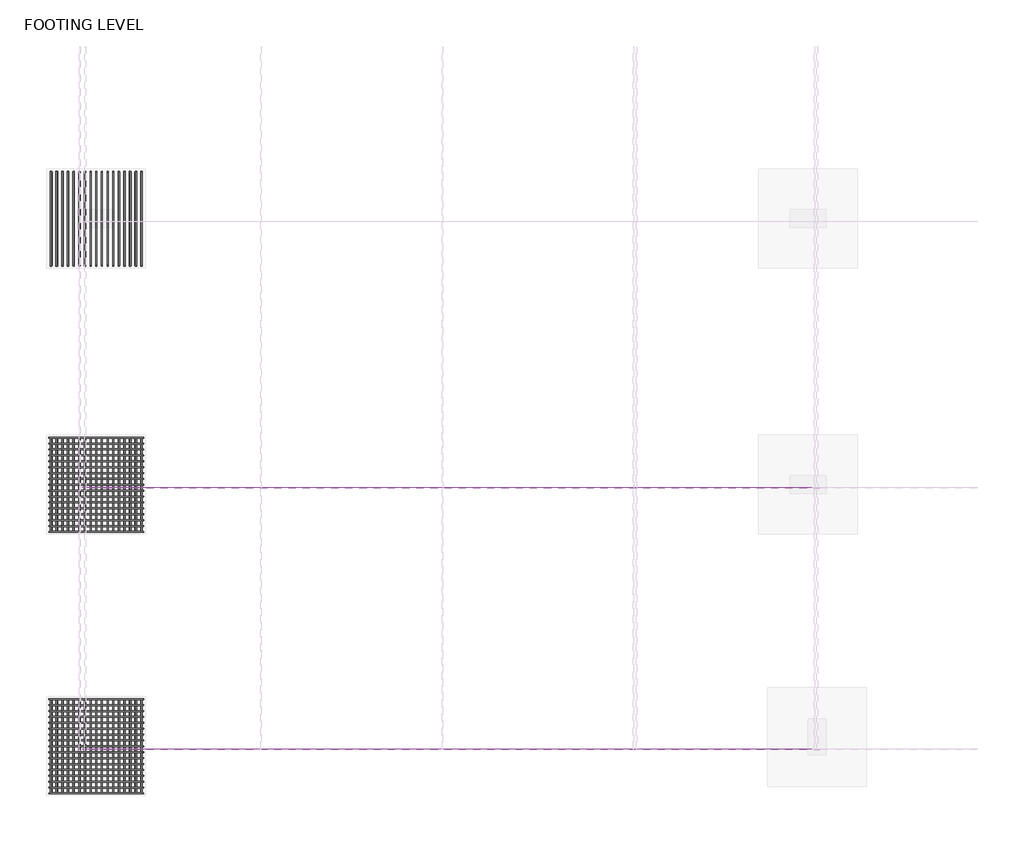
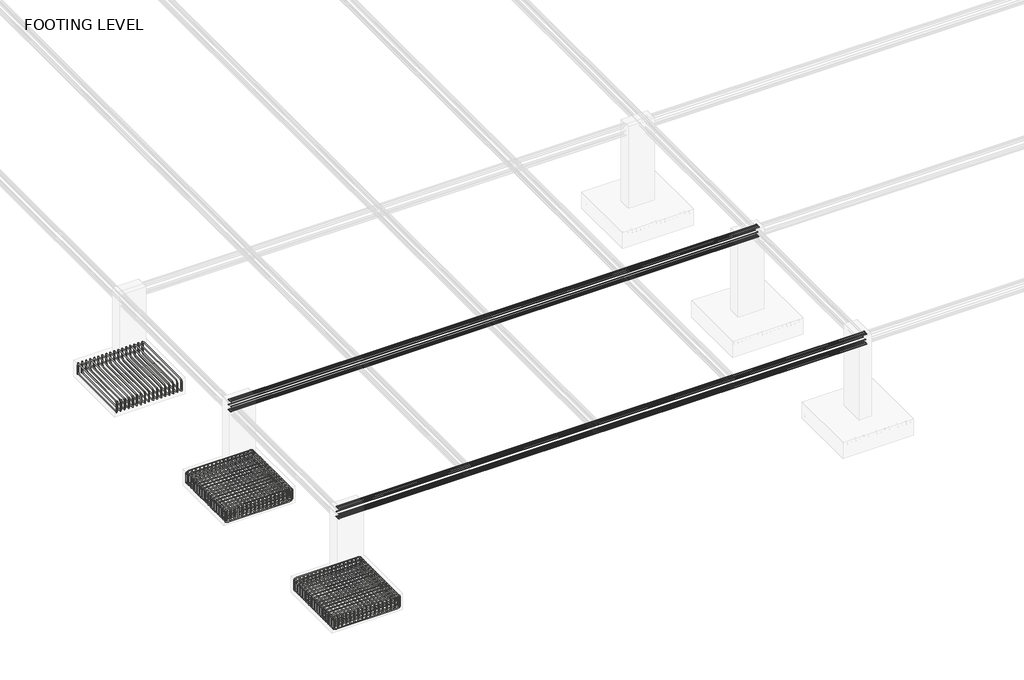
# One storey, part 3 of 19: 16 reinforcing bars.
"""IFC4 building model written with IfcOpenShell, lengths in millimetres."""

from ifc_helpers import new_model, si_unit, point, frame, origin, place, context, project, spatial, polyline, circle_curve, trimmed, segment, composite_curve, source, transform, mapped, element, save
from ifc_brep_helpers import swept_disk

model = new_model("IFC4")

# Units and contexts
model_context = context("Model", 3, world=origin())
ifc_project = project(units=[si_unit("LENGTHUNIT", "METRE", prefix="MILLI")], contexts=[model_context])

# Site, building, storey
site = spatial("IfcSite", under=ifc_project)
building = spatial("IfcBuilding", under=site)
storey = spatial("IfcBuildingStorey", under=building, Name="FOOTING LEVEL", Elevation=-3048.0)

# Reinforcing bars
placement = place(None, origin())
reinforcing_bar_shape = source(origin(), model_context, "Body", "SolidModel", [
    swept_disk(composite_curve([segment(polyline([(-17920.0723448, -29246.9205555, -3148.0), (-17920.0723448, -29246.9205555, -3470.1)]), True, "CONTINUOUS"), segment(trimmed(circle_curve(frame((-17920.0723448, -29156.7205555, -3470.1), z_axis=(1.0, 0.0, 0.0), x_axis=(0.0, -90.20000000000073, 0.0)), 90.2), [point((-17920.0723448, -29246.9205555, -3470.1))], [point((-17920.0723448, -29156.7205555, -3560.3))], True, "CARTESIAN"), True, "CONTINUOUS"), segment(polyline([(-17920.0723448, -29156.7205555, -3560.3), (-17920.0723448, -26962.5205555, -3560.3)]), True, "CONTINUOUS"), segment(trimmed(circle_curve(frame((-17920.0723448, -26962.5205555, -3470.1), z_axis=(1.0, 0.0, 0.0), x_axis=(0.0, 0.0, -90.20000000000027)), 90.2), [point((-17920.0723448, -26962.5205555, -3560.3))], [point((-17920.0723448, -26872.3205555, -3470.1))], True, "CARTESIAN"), True, "CONTINUOUS"), segment(polyline([(-17920.0723448, -26872.3205555, -3470.1), (-17920.0723448, -26872.3205555, -3148.0)]), True, "CONTINUOUS")], self_intersect=False), 12.7),
])
element("IfcReinforcingBar", 1, at=placement, inside=storey, context=model_context, shape_type="MappedRepresentation", body=[
    mapped(reinforcing_bar_shape, transform((0.0, 0.0, 0.0), x_axis=(1.0, 0.0, 0.0), y_axis=(0.0, 1.0, 0.0), z_axis=(0.0, 0.0, 1.0))),
    mapped(reinforcing_bar_shape, transform((140.8090411, 0.0, 0.0), x_axis=(1.0, 0.0, 0.0), y_axis=(0.0, 1.0, 0.0), z_axis=(0.0, 0.0, 1.0))),
    mapped(reinforcing_bar_shape, transform((281.6180821, 0.0, 0.0), x_axis=(1.0, 0.0, 0.0), y_axis=(0.0, 1.0, 0.0), z_axis=(0.0, 0.0, 1.0))),
    mapped(reinforcing_bar_shape, transform((422.4271232, 0.0, 0.0), x_axis=(1.0, 0.0, 0.0), y_axis=(0.0, 1.0, 0.0), z_axis=(0.0, 0.0, 1.0))),
    mapped(reinforcing_bar_shape, transform((563.2361643, 0.0, 0.0), x_axis=(1.0, 0.0, 0.0), y_axis=(0.0, 1.0, 0.0), z_axis=(0.0, 0.0, 1.0))),
    mapped(reinforcing_bar_shape, transform((704.0452054, 0.0, 0.0), x_axis=(1.0, 0.0, 0.0), y_axis=(0.0, 1.0, 0.0), z_axis=(0.0, 0.0, 1.0))),
    mapped(reinforcing_bar_shape, transform((844.8542464, 0.0, 0.0), x_axis=(1.0, 0.0, 0.0), y_axis=(0.0, 1.0, 0.0), z_axis=(0.0, 0.0, 1.0))),
    mapped(reinforcing_bar_shape, transform((985.6632875, 0.0, 0.0), x_axis=(1.0, 0.0, 0.0), y_axis=(0.0, 1.0, 0.0), z_axis=(0.0, 0.0, 1.0))),
    mapped(reinforcing_bar_shape, transform((1126.4723286, 0.0, 0.0), x_axis=(1.0, 0.0, 0.0), y_axis=(0.0, 1.0, 0.0), z_axis=(0.0, 0.0, 1.0))),
    mapped(reinforcing_bar_shape, transform((1267.2813697, 0.0, 0.0), x_axis=(1.0, 0.0, 0.0), y_axis=(0.0, 1.0, 0.0), z_axis=(0.0, 0.0, 1.0))),
    mapped(reinforcing_bar_shape, transform((1408.0904107, 0.0, 0.0), x_axis=(1.0, 0.0, 0.0), y_axis=(0.0, 1.0, 0.0), z_axis=(0.0, 0.0, 1.0))),
    mapped(reinforcing_bar_shape, transform((1548.8994518, 0.0, 0.0), x_axis=(1.0, 0.0, 0.0), y_axis=(0.0, 1.0, 0.0), z_axis=(0.0, 0.0, 1.0))),
    mapped(reinforcing_bar_shape, transform((1689.7084929, 0.0, 0.0), x_axis=(1.0, 0.0, 0.0), y_axis=(0.0, 1.0, 0.0), z_axis=(0.0, 0.0, 1.0))),
    mapped(reinforcing_bar_shape, transform((1830.517534, 0.0, 0.0), x_axis=(1.0, 0.0, 0.0), y_axis=(0.0, 1.0, 0.0), z_axis=(0.0, 0.0, 1.0))),
    mapped(reinforcing_bar_shape, transform((1971.326575, 0.0, 0.0), x_axis=(1.0, 0.0, 0.0), y_axis=(0.0, 1.0, 0.0), z_axis=(0.0, 0.0, 1.0))),
    mapped(reinforcing_bar_shape, transform((2112.1356161, 0.0, 0.0), x_axis=(1.0, 0.0, 0.0), y_axis=(0.0, 1.0, 0.0), z_axis=(0.0, 0.0, 1.0))),
    mapped(reinforcing_bar_shape, transform((2252.9446572, 0.0, 0.0), x_axis=(1.0, 0.0, 0.0), y_axis=(0.0, 1.0, 0.0), z_axis=(0.0, 0.0, 1.0))),
])
reinforcing_bar_2_shape = source(origin(), model_context, "Body", "SolidModel", [
    swept_disk(composite_curve([segment(polyline([(-15644.6802955, -29246.9205555, -3548.0), (-15644.6802955, -29246.9205555, -3225.9)]), True, "CONTINUOUS"), segment(trimmed(circle_curve(frame((-15644.6802955, -29156.7205555, -3225.9), z_axis=(-1.0, 0.0, 0.0), x_axis=(0.0, -90.20000000000073, 0.0)), 90.2), [point((-15644.6802955, -29246.9205555, -3225.9))], [point((-15644.6802955, -29156.7205555, -3135.7))], True, "CARTESIAN"), True, "CONTINUOUS"), segment(polyline([(-15644.6802955, -29156.7205555, -3135.7), (-15644.6802955, -26962.5205555, -3135.7)]), True, "CONTINUOUS"), segment(trimmed(circle_curve(frame((-15644.6802955, -26962.5205555, -3225.9), z_axis=(-1.0, 0.0, 0.0), x_axis=(0.0, 0.0, 90.20000000000027)), 90.2), [point((-15644.6802955, -26962.5205555, -3135.7))], [point((-15644.6802955, -26872.3205555, -3225.9))], True, "CARTESIAN"), True, "CONTINUOUS"), segment(polyline([(-15644.6802955, -26872.3205555, -3225.9), (-15644.6802955, -26872.3205555, -3548.0)]), True, "CONTINUOUS")], self_intersect=False), 12.7),
])
element("IfcReinforcingBar", 2, at=placement, inside=storey, context=model_context, shape_type="MappedRepresentation", body=[
    mapped(reinforcing_bar_2_shape, transform((0.0, 0.0, 0.0), x_axis=(1.0, 0.0, 0.0), y_axis=(0.0, 1.0, 0.0), z_axis=(0.0, 0.0, 1.0))),
    mapped(reinforcing_bar_2_shape, transform((-143.8496077, 0.0, 0.0), x_axis=(1.0, 0.0, 0.0), y_axis=(0.0, 1.0, 0.0), z_axis=(0.0, 0.0, 1.0))),
    mapped(reinforcing_bar_2_shape, transform((-287.6992155, 0.0, 0.0), x_axis=(1.0, 0.0, 0.0), y_axis=(0.0, 1.0, 0.0), z_axis=(0.0, 0.0, 1.0))),
    mapped(reinforcing_bar_2_shape, transform((-431.5488232, 0.0, 0.0), x_axis=(1.0, 0.0, 0.0), y_axis=(0.0, 1.0, 0.0), z_axis=(0.0, 0.0, 1.0))),
    mapped(reinforcing_bar_2_shape, transform((-575.398431, 0.0, 0.0), x_axis=(1.0, 0.0, 0.0), y_axis=(0.0, 1.0, 0.0), z_axis=(0.0, 0.0, 1.0))),
    mapped(reinforcing_bar_2_shape, transform((-719.2480387, 0.0, 0.0), x_axis=(1.0, 0.0, 0.0), y_axis=(0.0, 1.0, 0.0), z_axis=(0.0, 0.0, 1.0))),
    mapped(reinforcing_bar_2_shape, transform((-863.0976465, 0.0, 0.0), x_axis=(1.0, 0.0, 0.0), y_axis=(0.0, 1.0, 0.0), z_axis=(0.0, 0.0, 1.0))),
    mapped(reinforcing_bar_2_shape, transform((-1006.9472542, 0.0, 0.0), x_axis=(1.0, 0.0, 0.0), y_axis=(0.0, 1.0, 0.0), z_axis=(0.0, 0.0, 1.0))),
    mapped(reinforcing_bar_2_shape, transform((-1150.796862, 0.0, 0.0), x_axis=(1.0, 0.0, 0.0), y_axis=(0.0, 1.0, 0.0), z_axis=(0.0, 0.0, 1.0))),
    mapped(reinforcing_bar_2_shape, transform((-1294.6464697, 0.0, 0.0), x_axis=(1.0, 0.0, 0.0), y_axis=(0.0, 1.0, 0.0), z_axis=(0.0, 0.0, 1.0))),
    mapped(reinforcing_bar_2_shape, transform((-1438.4960775, 0.0, 0.0), x_axis=(1.0, 0.0, 0.0), y_axis=(0.0, 1.0, 0.0), z_axis=(0.0, 0.0, 1.0))),
    mapped(reinforcing_bar_2_shape, transform((-1582.3456852, 0.0, 0.0), x_axis=(1.0, 0.0, 0.0), y_axis=(0.0, 1.0, 0.0), z_axis=(0.0, 0.0, 1.0))),
    mapped(reinforcing_bar_2_shape, transform((-1726.195293, 0.0, 0.0), x_axis=(1.0, 0.0, 0.0), y_axis=(0.0, 1.0, 0.0), z_axis=(0.0, 0.0, 1.0))),
    mapped(reinforcing_bar_2_shape, transform((-1870.0449007, 0.0, 0.0), x_axis=(1.0, 0.0, 0.0), y_axis=(0.0, 1.0, 0.0), z_axis=(0.0, 0.0, 1.0))),
    mapped(reinforcing_bar_2_shape, transform((-2013.8945085, 0.0, 0.0), x_axis=(1.0, 0.0, 0.0), y_axis=(0.0, 1.0, 0.0), z_axis=(0.0, 0.0, 1.0))),
    mapped(reinforcing_bar_2_shape, transform((-2157.7441162, 0.0, 0.0), x_axis=(1.0, 0.0, 0.0), y_axis=(0.0, 1.0, 0.0), z_axis=(0.0, 0.0, 1.0))),
    mapped(reinforcing_bar_2_shape, transform((-2301.5937239, 0.0, 0.0), x_axis=(1.0, 0.0, 0.0), y_axis=(0.0, 1.0, 0.0), z_axis=(0.0, 0.0, 1.0))),
])
reinforcing_bar_3_shape = source(origin(), model_context, "Body", "SolidModel", [
    swept_disk(composite_curve([segment(polyline([(-17985.6412437, -26872.3205555, -3173.0), (-17985.6412437, -26872.3205555, -3495.1)]), True, "CONTINUOUS"), segment(trimmed(circle_curve(frame((-17895.4412437, -26872.3205555, -3495.1), z_axis=(0.0, -1.0, 0.0), x_axis=(-90.20000000000073, 0.0, 0.0)), 90.2), [point((-17985.6412437, -26872.3205555, -3495.1))], [point((-17895.4412437, -26872.3205555, -3585.3))], True, "CARTESIAN"), True, "CONTINUOUS"), segment(polyline([(-17895.4412437, -26872.3205555, -3585.3), (-15701.2412437, -26872.3205555, -3585.3)]), True, "CONTINUOUS"), segment(trimmed(circle_curve(frame((-15701.2412437, -26872.3205555, -3495.1), z_axis=(0.0, -1.0, 0.0), x_axis=(0.0, 0.0, -90.20000000000027)), 90.2), [point((-15701.2412437, -26872.3205555, -3585.3))], [point((-15611.0412437, -26872.3205555, -3495.1))], True, "CARTESIAN"), True, "CONTINUOUS"), segment(polyline([(-15611.0412437, -26872.3205555, -3495.1), (-15611.0412437, -26872.3205555, -3173.0)]), True, "CONTINUOUS")], self_intersect=False), 12.7),
])
element("IfcReinforcingBar", 3, at=placement, inside=storey, context=model_context, shape_type="MappedRepresentation", body=[
    mapped(reinforcing_bar_3_shape, transform((0.0, 0.0, 0.0), x_axis=(1.0, 0.0, 0.0), y_axis=(0.0, 1.0, 0.0), z_axis=(0.0, 0.0, 1.0))),
    mapped(reinforcing_bar_3_shape, transform((0.0, -148.4125, 0.0), x_axis=(1.0, 0.0, 0.0), y_axis=(0.0, 1.0, 0.0), z_axis=(0.0, 0.0, 1.0))),
    mapped(reinforcing_bar_3_shape, transform((0.0, -296.825, 0.0), x_axis=(1.0, 0.0, 0.0), y_axis=(0.0, 1.0, 0.0), z_axis=(0.0, 0.0, 1.0))),
    mapped(reinforcing_bar_3_shape, transform((0.0, -445.2375, 0.0), x_axis=(1.0, 0.0, 0.0), y_axis=(0.0, 1.0, 0.0), z_axis=(0.0, 0.0, 1.0))),
    mapped(reinforcing_bar_3_shape, transform((0.0, -593.65, 0.0), x_axis=(1.0, 0.0, 0.0), y_axis=(0.0, 1.0, 0.0), z_axis=(0.0, 0.0, 1.0))),
    mapped(reinforcing_bar_3_shape, transform((0.0, -742.0625, 0.0), x_axis=(1.0, 0.0, 0.0), y_axis=(0.0, 1.0, 0.0), z_axis=(0.0, 0.0, 1.0))),
    mapped(reinforcing_bar_3_shape, transform((0.0, -890.475, 0.0), x_axis=(1.0, 0.0, 0.0), y_axis=(0.0, 1.0, 0.0), z_axis=(0.0, 0.0, 1.0))),
    mapped(reinforcing_bar_3_shape, transform((0.0, -1038.8875, 0.0), x_axis=(1.0, 0.0, 0.0), y_axis=(0.0, 1.0, 0.0), z_axis=(0.0, 0.0, 1.0))),
    mapped(reinforcing_bar_3_shape, transform((0.0, -1187.3, 0.0), x_axis=(1.0, 0.0, 0.0), y_axis=(0.0, 1.0, 0.0), z_axis=(0.0, 0.0, 1.0))),
    mapped(reinforcing_bar_3_shape, transform((0.0, -1335.7125, 0.0), x_axis=(1.0, 0.0, 0.0), y_axis=(0.0, 1.0, 0.0), z_axis=(0.0, 0.0, 1.0))),
    mapped(reinforcing_bar_3_shape, transform((0.0, -1484.125, 0.0), x_axis=(1.0, 0.0, 0.0), y_axis=(0.0, 1.0, 0.0), z_axis=(0.0, 0.0, 1.0))),
    mapped(reinforcing_bar_3_shape, transform((0.0, -1632.5375, 0.0), x_axis=(1.0, 0.0, 0.0), y_axis=(0.0, 1.0, 0.0), z_axis=(0.0, 0.0, 1.0))),
    mapped(reinforcing_bar_3_shape, transform((0.0, -1780.95, 0.0), x_axis=(1.0, 0.0, 0.0), y_axis=(0.0, 1.0, 0.0), z_axis=(0.0, 0.0, 1.0))),
    mapped(reinforcing_bar_3_shape, transform((0.0, -1929.3625, 0.0), x_axis=(1.0, 0.0, 0.0), y_axis=(0.0, 1.0, 0.0), z_axis=(0.0, 0.0, 1.0))),
    mapped(reinforcing_bar_3_shape, transform((0.0, -2077.775, 0.0), x_axis=(1.0, 0.0, 0.0), y_axis=(0.0, 1.0, 0.0), z_axis=(0.0, 0.0, 1.0))),
    mapped(reinforcing_bar_3_shape, transform((0.0, -2226.1875, 0.0), x_axis=(1.0, 0.0, 0.0), y_axis=(0.0, 1.0, 0.0), z_axis=(0.0, 0.0, 1.0))),
    mapped(reinforcing_bar_3_shape, transform((0.0, -2374.6, 0.0), x_axis=(1.0, 0.0, 0.0), y_axis=(0.0, 1.0, 0.0), z_axis=(0.0, 0.0, 1.0))),
])
reinforcing_bar_4_shape = source(origin(), model_context, "Body", "SolidModel", [
    swept_disk(composite_curve([segment(polyline([(-15611.0412437, -26872.3205555, -3523.0), (-15611.0412437, -26872.3205555, -3200.9)]), True, "CONTINUOUS"), segment(trimmed(circle_curve(frame((-15701.2412437, -26872.3205555, -3200.9), z_axis=(0.0, -1.0, 0.0), x_axis=(90.20000000000073, 0.0, 0.0)), 90.2), [point((-15611.0412437, -26872.3205555, -3200.9))], [point((-15701.2412437, -26872.3205555, -3110.7))], True, "CARTESIAN"), True, "CONTINUOUS"), segment(polyline([(-15701.2412437, -26872.3205555, -3110.7), (-17895.4412437, -26872.3205555, -3110.7)]), True, "CONTINUOUS"), segment(trimmed(circle_curve(frame((-17895.4412437, -26872.3205555, -3200.9), z_axis=(0.0, -1.0, 0.0), x_axis=(0.0, 0.0, 90.20000000000027)), 90.2), [point((-17895.4412437, -26872.3205555, -3110.7))], [point((-17985.6412437, -26872.3205555, -3200.9))], True, "CARTESIAN"), True, "CONTINUOUS"), segment(polyline([(-17985.6412437, -26872.3205555, -3200.9), (-17985.6412437, -26872.3205555, -3523.0)]), True, "CONTINUOUS")], self_intersect=False), 12.7),
])
element("IfcReinforcingBar", 4, at=placement, inside=storey, context=model_context, shape_type="MappedRepresentation", body=[
    mapped(reinforcing_bar_4_shape, transform((0.0, 0.0, 0.0), x_axis=(1.0, 0.0, 0.0), y_axis=(0.0, 1.0, 0.0), z_axis=(0.0, 0.0, 1.0))),
    mapped(reinforcing_bar_4_shape, transform((0.0, -148.4125, 0.0), x_axis=(1.0, 0.0, 0.0), y_axis=(0.0, 1.0, 0.0), z_axis=(0.0, 0.0, 1.0))),
    mapped(reinforcing_bar_4_shape, transform((0.0, -296.825, 0.0), x_axis=(1.0, 0.0, 0.0), y_axis=(0.0, 1.0, 0.0), z_axis=(0.0, 0.0, 1.0))),
    mapped(reinforcing_bar_4_shape, transform((0.0, -445.2375, 0.0), x_axis=(1.0, 0.0, 0.0), y_axis=(0.0, 1.0, 0.0), z_axis=(0.0, 0.0, 1.0))),
    mapped(reinforcing_bar_4_shape, transform((0.0, -593.65, 0.0), x_axis=(1.0, 0.0, 0.0), y_axis=(0.0, 1.0, 0.0), z_axis=(0.0, 0.0, 1.0))),
    mapped(reinforcing_bar_4_shape, transform((0.0, -742.0625, 0.0), x_axis=(1.0, 0.0, 0.0), y_axis=(0.0, 1.0, 0.0), z_axis=(0.0, 0.0, 1.0))),
    mapped(reinforcing_bar_4_shape, transform((0.0, -890.475, 0.0), x_axis=(1.0, 0.0, 0.0), y_axis=(0.0, 1.0, 0.0), z_axis=(0.0, 0.0, 1.0))),
    mapped(reinforcing_bar_4_shape, transform((0.0, -1038.8875, 0.0), x_axis=(1.0, 0.0, 0.0), y_axis=(0.0, 1.0, 0.0), z_axis=(0.0, 0.0, 1.0))),
    mapped(reinforcing_bar_4_shape, transform((0.0, -1187.3, 0.0), x_axis=(1.0, 0.0, 0.0), y_axis=(0.0, 1.0, 0.0), z_axis=(0.0, 0.0, 1.0))),
    mapped(reinforcing_bar_4_shape, transform((0.0, -1335.7125, 0.0), x_axis=(1.0, 0.0, 0.0), y_axis=(0.0, 1.0, 0.0), z_axis=(0.0, 0.0, 1.0))),
    mapped(reinforcing_bar_4_shape, transform((0.0, -1484.125, 0.0), x_axis=(1.0, 0.0, 0.0), y_axis=(0.0, 1.0, 0.0), z_axis=(0.0, 0.0, 1.0))),
    mapped(reinforcing_bar_4_shape, transform((0.0, -1632.5375, 0.0), x_axis=(1.0, 0.0, 0.0), y_axis=(0.0, 1.0, 0.0), z_axis=(0.0, 0.0, 1.0))),
    mapped(reinforcing_bar_4_shape, transform((0.0, -1780.95, 0.0), x_axis=(1.0, 0.0, 0.0), y_axis=(0.0, 1.0, 0.0), z_axis=(0.0, 0.0, 1.0))),
    mapped(reinforcing_bar_4_shape, transform((0.0, -1929.3625, 0.0), x_axis=(1.0, 0.0, 0.0), y_axis=(0.0, 1.0, 0.0), z_axis=(0.0, 0.0, 1.0))),
    mapped(reinforcing_bar_4_shape, transform((0.0, -2077.775, 0.0), x_axis=(1.0, 0.0, 0.0), y_axis=(0.0, 1.0, 0.0), z_axis=(0.0, 0.0, 1.0))),
    mapped(reinforcing_bar_4_shape, transform((0.0, -2226.1875, 0.0), x_axis=(1.0, 0.0, 0.0), y_axis=(0.0, 1.0, 0.0), z_axis=(0.0, 0.0, 1.0))),
    mapped(reinforcing_bar_4_shape, transform((0.0, -2374.6, 0.0), x_axis=(1.0, 0.0, 0.0), y_axis=(0.0, 1.0, 0.0), z_axis=(0.0, 0.0, 1.0))),
])
reinforcing_bar_5_shape = source(origin(), model_context, "Body", "SolidModel", [
    swept_disk(composite_curve([segment(polyline([(-17920.0723448, -22655.6205555, -3148.0), (-17920.0723448, -22655.6205555, -3470.1)]), True, "CONTINUOUS"), segment(trimmed(circle_curve(frame((-17920.0723448, -22565.4205555, -3470.1), z_axis=(1.0, 0.0, 0.0), x_axis=(0.0, -90.20000000000073, 0.0)), 90.2), [point((-17920.0723448, -22655.6205555, -3470.1))], [point((-17920.0723448, -22565.4205555, -3560.3))], True, "CARTESIAN"), True, "CONTINUOUS"), segment(polyline([(-17920.0723448, -22565.4205555, -3560.3), (-17920.0723448, -20371.2205555, -3560.3)]), True, "CONTINUOUS"), segment(trimmed(circle_curve(frame((-17920.0723448, -20371.2205555, -3470.1), z_axis=(1.0, 0.0, 0.0), x_axis=(0.0, 0.0, -90.20000000000027)), 90.2), [point((-17920.0723448, -20371.2205555, -3560.3))], [point((-17920.0723448, -20281.0205555, -3470.1))], True, "CARTESIAN"), True, "CONTINUOUS"), segment(polyline([(-17920.0723448, -20281.0205555, -3470.1), (-17920.0723448, -20281.0205555, -3148.0)]), True, "CONTINUOUS")], self_intersect=False), 12.7),
])
element("IfcReinforcingBar", 5, at=placement, inside=storey, context=model_context, shape_type="MappedRepresentation", body=[
    mapped(reinforcing_bar_5_shape, transform((0.0, 0.0, 0.0), x_axis=(1.0, 0.0, 0.0), y_axis=(0.0, 1.0, 0.0), z_axis=(0.0, 0.0, 1.0))),
    mapped(reinforcing_bar_5_shape, transform((140.8090411, 0.0, 0.0), x_axis=(1.0, 0.0, 0.0), y_axis=(0.0, 1.0, 0.0), z_axis=(0.0, 0.0, 1.0))),
    mapped(reinforcing_bar_5_shape, transform((281.6180821, 0.0, 0.0), x_axis=(1.0, 0.0, 0.0), y_axis=(0.0, 1.0, 0.0), z_axis=(0.0, 0.0, 1.0))),
    mapped(reinforcing_bar_5_shape, transform((422.4271232, 0.0, 0.0), x_axis=(1.0, 0.0, 0.0), y_axis=(0.0, 1.0, 0.0), z_axis=(0.0, 0.0, 1.0))),
    mapped(reinforcing_bar_5_shape, transform((563.2361643, 0.0, 0.0), x_axis=(1.0, 0.0, 0.0), y_axis=(0.0, 1.0, 0.0), z_axis=(0.0, 0.0, 1.0))),
    mapped(reinforcing_bar_5_shape, transform((704.0452054, 0.0, 0.0), x_axis=(1.0, 0.0, 0.0), y_axis=(0.0, 1.0, 0.0), z_axis=(0.0, 0.0, 1.0))),
    mapped(reinforcing_bar_5_shape, transform((844.8542464, 0.0, 0.0), x_axis=(1.0, 0.0, 0.0), y_axis=(0.0, 1.0, 0.0), z_axis=(0.0, 0.0, 1.0))),
    mapped(reinforcing_bar_5_shape, transform((985.6632875, 0.0, 0.0), x_axis=(1.0, 0.0, 0.0), y_axis=(0.0, 1.0, 0.0), z_axis=(0.0, 0.0, 1.0))),
    mapped(reinforcing_bar_5_shape, transform((1126.4723286, 0.0, 0.0), x_axis=(1.0, 0.0, 0.0), y_axis=(0.0, 1.0, 0.0), z_axis=(0.0, 0.0, 1.0))),
    mapped(reinforcing_bar_5_shape, transform((1267.2813697, 0.0, 0.0), x_axis=(1.0, 0.0, 0.0), y_axis=(0.0, 1.0, 0.0), z_axis=(0.0, 0.0, 1.0))),
    mapped(reinforcing_bar_5_shape, transform((1408.0904107, 0.0, 0.0), x_axis=(1.0, 0.0, 0.0), y_axis=(0.0, 1.0, 0.0), z_axis=(0.0, 0.0, 1.0))),
    mapped(reinforcing_bar_5_shape, transform((1548.8994518, 0.0, 0.0), x_axis=(1.0, 0.0, 0.0), y_axis=(0.0, 1.0, 0.0), z_axis=(0.0, 0.0, 1.0))),
    mapped(reinforcing_bar_5_shape, transform((1689.7084929, 0.0, 0.0), x_axis=(1.0, 0.0, 0.0), y_axis=(0.0, 1.0, 0.0), z_axis=(0.0, 0.0, 1.0))),
    mapped(reinforcing_bar_5_shape, transform((1830.517534, 0.0, 0.0), x_axis=(1.0, 0.0, 0.0), y_axis=(0.0, 1.0, 0.0), z_axis=(0.0, 0.0, 1.0))),
    mapped(reinforcing_bar_5_shape, transform((1971.326575, 0.0, 0.0), x_axis=(1.0, 0.0, 0.0), y_axis=(0.0, 1.0, 0.0), z_axis=(0.0, 0.0, 1.0))),
    mapped(reinforcing_bar_5_shape, transform((2112.1356161, 0.0, 0.0), x_axis=(1.0, 0.0, 0.0), y_axis=(0.0, 1.0, 0.0), z_axis=(0.0, 0.0, 1.0))),
    mapped(reinforcing_bar_5_shape, transform((2252.9446572, 0.0, 0.0), x_axis=(1.0, 0.0, 0.0), y_axis=(0.0, 1.0, 0.0), z_axis=(0.0, 0.0, 1.0))),
])
reinforcing_bar_6_shape = source(origin(), model_context, "Body", "SolidModel", [
    swept_disk(composite_curve([segment(polyline([(-15644.6802955, -22655.6205555, -3548.0), (-15644.6802955, -22655.6205555, -3225.9)]), True, "CONTINUOUS"), segment(trimmed(circle_curve(frame((-15644.6802955, -22565.4205555, -3225.9), z_axis=(-1.0, 0.0, 0.0), x_axis=(0.0, -90.20000000000073, 0.0)), 90.2), [point((-15644.6802955, -22655.6205555, -3225.9))], [point((-15644.6802955, -22565.4205555, -3135.7))], True, "CARTESIAN"), True, "CONTINUOUS"), segment(polyline([(-15644.6802955, -22565.4205555, -3135.7), (-15644.6802955, -20371.2205555, -3135.7)]), True, "CONTINUOUS"), segment(trimmed(circle_curve(frame((-15644.6802955, -20371.2205555, -3225.9), z_axis=(-1.0, 0.0, 0.0), x_axis=(0.0, 0.0, 90.20000000000027)), 90.2), [point((-15644.6802955, -20371.2205555, -3135.7))], [point((-15644.6802955, -20281.0205555, -3225.9))], True, "CARTESIAN"), True, "CONTINUOUS"), segment(polyline([(-15644.6802955, -20281.0205555, -3225.9), (-15644.6802955, -20281.0205555, -3548.0)]), True, "CONTINUOUS")], self_intersect=False), 12.7),
])
element("IfcReinforcingBar", 6, at=placement, inside=storey, context=model_context, shape_type="MappedRepresentation", body=[
    mapped(reinforcing_bar_6_shape, transform((0.0, 0.0, 0.0), x_axis=(1.0, 0.0, 0.0), y_axis=(0.0, 1.0, 0.0), z_axis=(0.0, 0.0, 1.0))),
    mapped(reinforcing_bar_6_shape, transform((-143.8496077, 0.0, 0.0), x_axis=(1.0, 0.0, 0.0), y_axis=(0.0, 1.0, 0.0), z_axis=(0.0, 0.0, 1.0))),
    mapped(reinforcing_bar_6_shape, transform((-287.6992155, 0.0, 0.0), x_axis=(1.0, 0.0, 0.0), y_axis=(0.0, 1.0, 0.0), z_axis=(0.0, 0.0, 1.0))),
    mapped(reinforcing_bar_6_shape, transform((-431.5488232, 0.0, 0.0), x_axis=(1.0, 0.0, 0.0), y_axis=(0.0, 1.0, 0.0), z_axis=(0.0, 0.0, 1.0))),
    mapped(reinforcing_bar_6_shape, transform((-575.398431, 0.0, 0.0), x_axis=(1.0, 0.0, 0.0), y_axis=(0.0, 1.0, 0.0), z_axis=(0.0, 0.0, 1.0))),
    mapped(reinforcing_bar_6_shape, transform((-719.2480387, 0.0, 0.0), x_axis=(1.0, 0.0, 0.0), y_axis=(0.0, 1.0, 0.0), z_axis=(0.0, 0.0, 1.0))),
    mapped(reinforcing_bar_6_shape, transform((-863.0976465, 0.0, 0.0), x_axis=(1.0, 0.0, 0.0), y_axis=(0.0, 1.0, 0.0), z_axis=(0.0, 0.0, 1.0))),
    mapped(reinforcing_bar_6_shape, transform((-1006.9472542, 0.0, 0.0), x_axis=(1.0, 0.0, 0.0), y_axis=(0.0, 1.0, 0.0), z_axis=(0.0, 0.0, 1.0))),
    mapped(reinforcing_bar_6_shape, transform((-1150.796862, 0.0, 0.0), x_axis=(1.0, 0.0, 0.0), y_axis=(0.0, 1.0, 0.0), z_axis=(0.0, 0.0, 1.0))),
    mapped(reinforcing_bar_6_shape, transform((-1294.6464697, 0.0, 0.0), x_axis=(1.0, 0.0, 0.0), y_axis=(0.0, 1.0, 0.0), z_axis=(0.0, 0.0, 1.0))),
    mapped(reinforcing_bar_6_shape, transform((-1438.4960775, 0.0, 0.0), x_axis=(1.0, 0.0, 0.0), y_axis=(0.0, 1.0, 0.0), z_axis=(0.0, 0.0, 1.0))),
    mapped(reinforcing_bar_6_shape, transform((-1582.3456852, 0.0, 0.0), x_axis=(1.0, 0.0, 0.0), y_axis=(0.0, 1.0, 0.0), z_axis=(0.0, 0.0, 1.0))),
    mapped(reinforcing_bar_6_shape, transform((-1726.195293, 0.0, 0.0), x_axis=(1.0, 0.0, 0.0), y_axis=(0.0, 1.0, 0.0), z_axis=(0.0, 0.0, 1.0))),
    mapped(reinforcing_bar_6_shape, transform((-1870.0449007, 0.0, 0.0), x_axis=(1.0, 0.0, 0.0), y_axis=(0.0, 1.0, 0.0), z_axis=(0.0, 0.0, 1.0))),
    mapped(reinforcing_bar_6_shape, transform((-2013.8945085, 0.0, 0.0), x_axis=(1.0, 0.0, 0.0), y_axis=(0.0, 1.0, 0.0), z_axis=(0.0, 0.0, 1.0))),
    mapped(reinforcing_bar_6_shape, transform((-2157.7441162, 0.0, 0.0), x_axis=(1.0, 0.0, 0.0), y_axis=(0.0, 1.0, 0.0), z_axis=(0.0, 0.0, 1.0))),
    mapped(reinforcing_bar_6_shape, transform((-2301.5937239, 0.0, 0.0), x_axis=(1.0, 0.0, 0.0), y_axis=(0.0, 1.0, 0.0), z_axis=(0.0, 0.0, 1.0))),
])
reinforcing_bar_7_shape = source(origin(), model_context, "Body", "SolidModel", [
    swept_disk(composite_curve([segment(polyline([(-17985.6412437, -20281.0205555, -3173.0), (-17985.6412437, -20281.0205555, -3495.1)]), True, "CONTINUOUS"), segment(trimmed(circle_curve(frame((-17895.4412437, -20281.0205555, -3495.1), z_axis=(0.0, -1.0, 0.0), x_axis=(-90.20000000000073, 0.0, 0.0)), 90.2), [point((-17985.6412437, -20281.0205555, -3495.1))], [point((-17895.4412437, -20281.0205555, -3585.3))], True, "CARTESIAN"), True, "CONTINUOUS"), segment(polyline([(-17895.4412437, -20281.0205555, -3585.3), (-15701.2412437, -20281.0205555, -3585.3)]), True, "CONTINUOUS"), segment(trimmed(circle_curve(frame((-15701.2412437, -20281.0205555, -3495.1), z_axis=(0.0, -1.0, 0.0), x_axis=(0.0, 0.0, -90.20000000000027)), 90.2), [point((-15701.2412437, -20281.0205555, -3585.3))], [point((-15611.0412437, -20281.0205555, -3495.1))], True, "CARTESIAN"), True, "CONTINUOUS"), segment(polyline([(-15611.0412437, -20281.0205555, -3495.1), (-15611.0412437, -20281.0205555, -3173.0)]), True, "CONTINUOUS")], self_intersect=False), 12.7),
])
element("IfcReinforcingBar", 7, at=placement, inside=storey, context=model_context, shape_type="MappedRepresentation", body=[
    mapped(reinforcing_bar_7_shape, transform((0.0, 0.0, 0.0), x_axis=(1.0, 0.0, 0.0), y_axis=(0.0, 1.0, 0.0), z_axis=(0.0, 0.0, 1.0))),
    mapped(reinforcing_bar_7_shape, transform((0.0, -148.4125, 0.0), x_axis=(1.0, 0.0, 0.0), y_axis=(0.0, 1.0, 0.0), z_axis=(0.0, 0.0, 1.0))),
    mapped(reinforcing_bar_7_shape, transform((0.0, -296.825, 0.0), x_axis=(1.0, 0.0, 0.0), y_axis=(0.0, 1.0, 0.0), z_axis=(0.0, 0.0, 1.0))),
    mapped(reinforcing_bar_7_shape, transform((0.0, -445.2375, 0.0), x_axis=(1.0, 0.0, 0.0), y_axis=(0.0, 1.0, 0.0), z_axis=(0.0, 0.0, 1.0))),
    mapped(reinforcing_bar_7_shape, transform((0.0, -593.65, 0.0), x_axis=(1.0, 0.0, 0.0), y_axis=(0.0, 1.0, 0.0), z_axis=(0.0, 0.0, 1.0))),
    mapped(reinforcing_bar_7_shape, transform((0.0, -742.0625, 0.0), x_axis=(1.0, 0.0, 0.0), y_axis=(0.0, 1.0, 0.0), z_axis=(0.0, 0.0, 1.0))),
    mapped(reinforcing_bar_7_shape, transform((0.0, -890.475, 0.0), x_axis=(1.0, 0.0, 0.0), y_axis=(0.0, 1.0, 0.0), z_axis=(0.0, 0.0, 1.0))),
    mapped(reinforcing_bar_7_shape, transform((0.0, -1038.8875, 0.0), x_axis=(1.0, 0.0, 0.0), y_axis=(0.0, 1.0, 0.0), z_axis=(0.0, 0.0, 1.0))),
    mapped(reinforcing_bar_7_shape, transform((0.0, -1187.3, 0.0), x_axis=(1.0, 0.0, 0.0), y_axis=(0.0, 1.0, 0.0), z_axis=(0.0, 0.0, 1.0))),
    mapped(reinforcing_bar_7_shape, transform((0.0, -1335.7125, 0.0), x_axis=(1.0, 0.0, 0.0), y_axis=(0.0, 1.0, 0.0), z_axis=(0.0, 0.0, 1.0))),
    mapped(reinforcing_bar_7_shape, transform((0.0, -1484.125, 0.0), x_axis=(1.0, 0.0, 0.0), y_axis=(0.0, 1.0, 0.0), z_axis=(0.0, 0.0, 1.0))),
    mapped(reinforcing_bar_7_shape, transform((0.0, -1632.5375, 0.0), x_axis=(1.0, 0.0, 0.0), y_axis=(0.0, 1.0, 0.0), z_axis=(0.0, 0.0, 1.0))),
    mapped(reinforcing_bar_7_shape, transform((0.0, -1780.95, 0.0), x_axis=(1.0, 0.0, 0.0), y_axis=(0.0, 1.0, 0.0), z_axis=(0.0, 0.0, 1.0))),
    mapped(reinforcing_bar_7_shape, transform((0.0, -1929.3625, 0.0), x_axis=(1.0, 0.0, 0.0), y_axis=(0.0, 1.0, 0.0), z_axis=(0.0, 0.0, 1.0))),
    mapped(reinforcing_bar_7_shape, transform((0.0, -2077.775, 0.0), x_axis=(1.0, 0.0, 0.0), y_axis=(0.0, 1.0, 0.0), z_axis=(0.0, 0.0, 1.0))),
    mapped(reinforcing_bar_7_shape, transform((0.0, -2226.1875, 0.0), x_axis=(1.0, 0.0, 0.0), y_axis=(0.0, 1.0, 0.0), z_axis=(0.0, 0.0, 1.0))),
    mapped(reinforcing_bar_7_shape, transform((0.0, -2374.6, 0.0), x_axis=(1.0, 0.0, 0.0), y_axis=(0.0, 1.0, 0.0), z_axis=(0.0, 0.0, 1.0))),
])
reinforcing_bar_8_shape = source(origin(), model_context, "Body", "SolidModel", [
    swept_disk(composite_curve([segment(polyline([(-15611.0412437, -20281.0205555, -3523.0), (-15611.0412437, -20281.0205555, -3200.9)]), True, "CONTINUOUS"), segment(trimmed(circle_curve(frame((-15701.2412437, -20281.0205555, -3200.9), z_axis=(0.0, -1.0, 0.0), x_axis=(90.20000000000073, 0.0, 0.0)), 90.2), [point((-15611.0412437, -20281.0205555, -3200.9))], [point((-15701.2412437, -20281.0205555, -3110.7))], True, "CARTESIAN"), True, "CONTINUOUS"), segment(polyline([(-15701.2412437, -20281.0205555, -3110.7), (-17895.4412437, -20281.0205555, -3110.7)]), True, "CONTINUOUS"), segment(trimmed(circle_curve(frame((-17895.4412437, -20281.0205555, -3200.9), z_axis=(0.0, -1.0, 0.0), x_axis=(0.0, 0.0, 90.20000000000027)), 90.2), [point((-17895.4412437, -20281.0205555, -3110.7))], [point((-17985.6412437, -20281.0205555, -3200.9))], True, "CARTESIAN"), True, "CONTINUOUS"), segment(polyline([(-17985.6412437, -20281.0205555, -3200.9), (-17985.6412437, -20281.0205555, -3523.0)]), True, "CONTINUOUS")], self_intersect=False), 12.7),
])
element("IfcReinforcingBar", 8, at=placement, inside=storey, context=model_context, shape_type="MappedRepresentation", body=[
    mapped(reinforcing_bar_8_shape, transform((0.0, 0.0, 0.0), x_axis=(1.0, 0.0, 0.0), y_axis=(0.0, 1.0, 0.0), z_axis=(0.0, 0.0, 1.0))),
    mapped(reinforcing_bar_8_shape, transform((0.0, -148.4125, 0.0), x_axis=(1.0, 0.0, 0.0), y_axis=(0.0, 1.0, 0.0), z_axis=(0.0, 0.0, 1.0))),
    mapped(reinforcing_bar_8_shape, transform((0.0, -296.825, 0.0), x_axis=(1.0, 0.0, 0.0), y_axis=(0.0, 1.0, 0.0), z_axis=(0.0, 0.0, 1.0))),
    mapped(reinforcing_bar_8_shape, transform((0.0, -445.2375, 0.0), x_axis=(1.0, 0.0, 0.0), y_axis=(0.0, 1.0, 0.0), z_axis=(0.0, 0.0, 1.0))),
    mapped(reinforcing_bar_8_shape, transform((0.0, -593.65, 0.0), x_axis=(1.0, 0.0, 0.0), y_axis=(0.0, 1.0, 0.0), z_axis=(0.0, 0.0, 1.0))),
    mapped(reinforcing_bar_8_shape, transform((0.0, -742.0625, 0.0), x_axis=(1.0, 0.0, 0.0), y_axis=(0.0, 1.0, 0.0), z_axis=(0.0, 0.0, 1.0))),
    mapped(reinforcing_bar_8_shape, transform((0.0, -890.475, 0.0), x_axis=(1.0, 0.0, 0.0), y_axis=(0.0, 1.0, 0.0), z_axis=(0.0, 0.0, 1.0))),
    mapped(reinforcing_bar_8_shape, transform((0.0, -1038.8875, 0.0), x_axis=(1.0, 0.0, 0.0), y_axis=(0.0, 1.0, 0.0), z_axis=(0.0, 0.0, 1.0))),
    mapped(reinforcing_bar_8_shape, transform((0.0, -1187.3, 0.0), x_axis=(1.0, 0.0, 0.0), y_axis=(0.0, 1.0, 0.0), z_axis=(0.0, 0.0, 1.0))),
    mapped(reinforcing_bar_8_shape, transform((0.0, -1335.7125, 0.0), x_axis=(1.0, 0.0, 0.0), y_axis=(0.0, 1.0, 0.0), z_axis=(0.0, 0.0, 1.0))),
    mapped(reinforcing_bar_8_shape, transform((0.0, -1484.125, 0.0), x_axis=(1.0, 0.0, 0.0), y_axis=(0.0, 1.0, 0.0), z_axis=(0.0, 0.0, 1.0))),
    mapped(reinforcing_bar_8_shape, transform((0.0, -1632.5375, 0.0), x_axis=(1.0, 0.0, 0.0), y_axis=(0.0, 1.0, 0.0), z_axis=(0.0, 0.0, 1.0))),
    mapped(reinforcing_bar_8_shape, transform((0.0, -1780.95, 0.0), x_axis=(1.0, 0.0, 0.0), y_axis=(0.0, 1.0, 0.0), z_axis=(0.0, 0.0, 1.0))),
    mapped(reinforcing_bar_8_shape, transform((0.0, -1929.3625, 0.0), x_axis=(1.0, 0.0, 0.0), y_axis=(0.0, 1.0, 0.0), z_axis=(0.0, 0.0, 1.0))),
    mapped(reinforcing_bar_8_shape, transform((0.0, -2077.775, 0.0), x_axis=(1.0, 0.0, 0.0), y_axis=(0.0, 1.0, 0.0), z_axis=(0.0, 0.0, 1.0))),
    mapped(reinforcing_bar_8_shape, transform((0.0, -2226.1875, 0.0), x_axis=(1.0, 0.0, 0.0), y_axis=(0.0, 1.0, 0.0), z_axis=(0.0, 0.0, 1.0))),
    mapped(reinforcing_bar_8_shape, transform((0.0, -2374.6, 0.0), x_axis=(1.0, 0.0, 0.0), y_axis=(0.0, 1.0, 0.0), z_axis=(0.0, 0.0, 1.0))),
])
reinforcing_bar_9_shape = source(origin(), model_context, "Body", "SolidModel", [
    swept_disk(composite_curve([segment(polyline([(-17920.0723448, -15950.0205555, -3148.0), (-17920.0723448, -15950.0205555, -3470.1)]), True, "CONTINUOUS"), segment(trimmed(circle_curve(frame((-17920.0723448, -15859.8205555, -3470.1), z_axis=(1.0, 0.0, 0.0), x_axis=(0.0, -90.19999999999891, 0.0)), 90.2), [point((-17920.0723448, -15950.0205555, -3470.1))], [point((-17920.0723448, -15859.8205555, -3560.3))], True, "CARTESIAN"), True, "CONTINUOUS"), segment(polyline([(-17920.0723448, -15859.8205555, -3560.3), (-17920.0723448, -13665.6205555, -3560.3)]), True, "CONTINUOUS"), segment(trimmed(circle_curve(frame((-17920.0723448, -13665.6205555, -3470.1), z_axis=(1.0, 0.0, 0.0), x_axis=(0.0, 0.0, -90.20000000000027)), 90.2), [point((-17920.0723448, -13665.6205555, -3560.3))], [point((-17920.0723448, -13575.4205555, -3470.1))], True, "CARTESIAN"), True, "CONTINUOUS"), segment(polyline([(-17920.0723448, -13575.4205555, -3470.1), (-17920.0723448, -13575.4205555, -3148.0)]), True, "CONTINUOUS")], self_intersect=False), 12.7),
])
element("IfcReinforcingBar", 9, at=placement, inside=storey, context=model_context, shape_type="MappedRepresentation", body=[
    mapped(reinforcing_bar_9_shape, transform((0.0, 0.0, 0.0), x_axis=(1.0, 0.0, 0.0), y_axis=(0.0, 1.0, 0.0), z_axis=(0.0, 0.0, 1.0))),
    mapped(reinforcing_bar_9_shape, transform((140.8090411, 0.0, 0.0), x_axis=(1.0, 0.0, 0.0), y_axis=(0.0, 1.0, 0.0), z_axis=(0.0, 0.0, 1.0))),
    mapped(reinforcing_bar_9_shape, transform((281.6180821, 0.0, 0.0), x_axis=(1.0, 0.0, 0.0), y_axis=(0.0, 1.0, 0.0), z_axis=(0.0, 0.0, 1.0))),
    mapped(reinforcing_bar_9_shape, transform((422.4271232, 0.0, 0.0), x_axis=(1.0, 0.0, 0.0), y_axis=(0.0, 1.0, 0.0), z_axis=(0.0, 0.0, 1.0))),
    mapped(reinforcing_bar_9_shape, transform((563.2361643, 0.0, 0.0), x_axis=(1.0, 0.0, 0.0), y_axis=(0.0, 1.0, 0.0), z_axis=(0.0, 0.0, 1.0))),
    mapped(reinforcing_bar_9_shape, transform((704.0452054, 0.0, 0.0), x_axis=(1.0, 0.0, 0.0), y_axis=(0.0, 1.0, 0.0), z_axis=(0.0, 0.0, 1.0))),
    mapped(reinforcing_bar_9_shape, transform((844.8542464, 0.0, 0.0), x_axis=(1.0, 0.0, 0.0), y_axis=(0.0, 1.0, 0.0), z_axis=(0.0, 0.0, 1.0))),
    mapped(reinforcing_bar_9_shape, transform((985.6632875, 0.0, 0.0), x_axis=(1.0, 0.0, 0.0), y_axis=(0.0, 1.0, 0.0), z_axis=(0.0, 0.0, 1.0))),
    mapped(reinforcing_bar_9_shape, transform((1126.4723286, 0.0, 0.0), x_axis=(1.0, 0.0, 0.0), y_axis=(0.0, 1.0, 0.0), z_axis=(0.0, 0.0, 1.0))),
    mapped(reinforcing_bar_9_shape, transform((1267.2813697, 0.0, 0.0), x_axis=(1.0, 0.0, 0.0), y_axis=(0.0, 1.0, 0.0), z_axis=(0.0, 0.0, 1.0))),
    mapped(reinforcing_bar_9_shape, transform((1408.0904107, 0.0, 0.0), x_axis=(1.0, 0.0, 0.0), y_axis=(0.0, 1.0, 0.0), z_axis=(0.0, 0.0, 1.0))),
    mapped(reinforcing_bar_9_shape, transform((1548.8994518, 0.0, 0.0), x_axis=(1.0, 0.0, 0.0), y_axis=(0.0, 1.0, 0.0), z_axis=(0.0, 0.0, 1.0))),
    mapped(reinforcing_bar_9_shape, transform((1689.7084929, 0.0, 0.0), x_axis=(1.0, 0.0, 0.0), y_axis=(0.0, 1.0, 0.0), z_axis=(0.0, 0.0, 1.0))),
    mapped(reinforcing_bar_9_shape, transform((1830.517534, 0.0, 0.0), x_axis=(1.0, 0.0, 0.0), y_axis=(0.0, 1.0, 0.0), z_axis=(0.0, 0.0, 1.0))),
    mapped(reinforcing_bar_9_shape, transform((1971.326575, 0.0, 0.0), x_axis=(1.0, 0.0, 0.0), y_axis=(0.0, 1.0, 0.0), z_axis=(0.0, 0.0, 1.0))),
    mapped(reinforcing_bar_9_shape, transform((2112.1356161, 0.0, 0.0), x_axis=(1.0, 0.0, 0.0), y_axis=(0.0, 1.0, 0.0), z_axis=(0.0, 0.0, 1.0))),
    mapped(reinforcing_bar_9_shape, transform((2252.9446572, 0.0, 0.0), x_axis=(1.0, 0.0, 0.0), y_axis=(0.0, 1.0, 0.0), z_axis=(0.0, 0.0, 1.0))),
])
reinforcing_bar_10_shape = source(origin(), model_context, "Body", "SolidModel", [
    swept_disk(composite_curve([segment(polyline([(-15644.6802955, -15950.0205555, -3548.0), (-15644.6802955, -15950.0205555, -3225.9)]), True, "CONTINUOUS"), segment(trimmed(circle_curve(frame((-15644.6802955, -15859.8205555, -3225.9), z_axis=(-1.0, 0.0, 0.0), x_axis=(0.0, -90.19999999999891, 0.0)), 90.2), [point((-15644.6802955, -15950.0205555, -3225.9))], [point((-15644.6802955, -15859.8205555, -3135.7))], True, "CARTESIAN"), True, "CONTINUOUS"), segment(polyline([(-15644.6802955, -15859.8205555, -3135.7), (-15644.6802955, -13665.6205555, -3135.7)]), True, "CONTINUOUS"), segment(trimmed(circle_curve(frame((-15644.6802955, -13665.6205555, -3225.9), z_axis=(-1.0, 0.0, 0.0), x_axis=(0.0, 0.0, 90.20000000000027)), 90.2), [point((-15644.6802955, -13665.6205555, -3135.7))], [point((-15644.6802955, -13575.4205555, -3225.9))], True, "CARTESIAN"), True, "CONTINUOUS"), segment(polyline([(-15644.6802955, -13575.4205555, -3225.9), (-15644.6802955, -13575.4205555, -3548.0)]), True, "CONTINUOUS")], self_intersect=False), 12.7),
])
element("IfcReinforcingBar", 10, at=placement, inside=storey, context=model_context, shape_type="MappedRepresentation", body=[
    mapped(reinforcing_bar_10_shape, transform((0.0, 0.0, 0.0), x_axis=(1.0, 0.0, 0.0), y_axis=(0.0, 1.0, 0.0), z_axis=(0.0, 0.0, 1.0))),
    mapped(reinforcing_bar_10_shape, transform((-143.8496077, 0.0, 0.0), x_axis=(1.0, 0.0, 0.0), y_axis=(0.0, 1.0, 0.0), z_axis=(0.0, 0.0, 1.0))),
    mapped(reinforcing_bar_10_shape, transform((-287.6992155, 0.0, 0.0), x_axis=(1.0, 0.0, 0.0), y_axis=(0.0, 1.0, 0.0), z_axis=(0.0, 0.0, 1.0))),
    mapped(reinforcing_bar_10_shape, transform((-431.5488232, 0.0, 0.0), x_axis=(1.0, 0.0, 0.0), y_axis=(0.0, 1.0, 0.0), z_axis=(0.0, 0.0, 1.0))),
    mapped(reinforcing_bar_10_shape, transform((-575.398431, 0.0, 0.0), x_axis=(1.0, 0.0, 0.0), y_axis=(0.0, 1.0, 0.0), z_axis=(0.0, 0.0, 1.0))),
    mapped(reinforcing_bar_10_shape, transform((-719.2480387, 0.0, 0.0), x_axis=(1.0, 0.0, 0.0), y_axis=(0.0, 1.0, 0.0), z_axis=(0.0, 0.0, 1.0))),
    mapped(reinforcing_bar_10_shape, transform((-863.0976465, 0.0, 0.0), x_axis=(1.0, 0.0, 0.0), y_axis=(0.0, 1.0, 0.0), z_axis=(0.0, 0.0, 1.0))),
    mapped(reinforcing_bar_10_shape, transform((-1006.9472542, 0.0, 0.0), x_axis=(1.0, 0.0, 0.0), y_axis=(0.0, 1.0, 0.0), z_axis=(0.0, 0.0, 1.0))),
    mapped(reinforcing_bar_10_shape, transform((-1150.796862, 0.0, 0.0), x_axis=(1.0, 0.0, 0.0), y_axis=(0.0, 1.0, 0.0), z_axis=(0.0, 0.0, 1.0))),
    mapped(reinforcing_bar_10_shape, transform((-1294.6464697, 0.0, 0.0), x_axis=(1.0, 0.0, 0.0), y_axis=(0.0, 1.0, 0.0), z_axis=(0.0, 0.0, 1.0))),
    mapped(reinforcing_bar_10_shape, transform((-1438.4960775, 0.0, 0.0), x_axis=(1.0, 0.0, 0.0), y_axis=(0.0, 1.0, 0.0), z_axis=(0.0, 0.0, 1.0))),
    mapped(reinforcing_bar_10_shape, transform((-1582.3456852, 0.0, 0.0), x_axis=(1.0, 0.0, 0.0), y_axis=(0.0, 1.0, 0.0), z_axis=(0.0, 0.0, 1.0))),
    mapped(reinforcing_bar_10_shape, transform((-1726.195293, 0.0, 0.0), x_axis=(1.0, 0.0, 0.0), y_axis=(0.0, 1.0, 0.0), z_axis=(0.0, 0.0, 1.0))),
    mapped(reinforcing_bar_10_shape, transform((-1870.0449007, 0.0, 0.0), x_axis=(1.0, 0.0, 0.0), y_axis=(0.0, 1.0, 0.0), z_axis=(0.0, 0.0, 1.0))),
    mapped(reinforcing_bar_10_shape, transform((-2013.8945085, 0.0, 0.0), x_axis=(1.0, 0.0, 0.0), y_axis=(0.0, 1.0, 0.0), z_axis=(0.0, 0.0, 1.0))),
    mapped(reinforcing_bar_10_shape, transform((-2157.7441162, 0.0, 0.0), x_axis=(1.0, 0.0, 0.0), y_axis=(0.0, 1.0, 0.0), z_axis=(0.0, 0.0, 1.0))),
    mapped(reinforcing_bar_10_shape, transform((-2301.5937239, 0.0, 0.0), x_axis=(1.0, 0.0, 0.0), y_axis=(0.0, 1.0, 0.0), z_axis=(0.0, 0.0, 1.0))),
])
reinforcing_bar_11_shape = source(origin(), model_context, "Body", "SolidModel", [
    swept_disk(composite_curve([segment(polyline([(1507.3728755, -27989.7999188, -412.7206367), (-17142.0118379, -27989.7999188, -412.7206367)]), True, "CONTINUOUS")], self_intersect=False), 7.95),
])
element("IfcReinforcingBar", 11, at=placement, inside=storey, context=model_context, shape_type="MappedRepresentation", body=[
    mapped(reinforcing_bar_11_shape, transform((0.0, 0.0, 0.0), x_axis=(1.0, 0.0, 0.0), y_axis=(0.0, 1.0, 0.0), z_axis=(0.0, 0.0, 1.0))),
    mapped(reinforcing_bar_11_shape, transform((0.0, -69.8206367, 0.0), x_axis=(1.0, 0.0, 0.0), y_axis=(0.0, 1.0, 0.0), z_axis=(0.0, 0.0, 1.0))),
    mapped(reinforcing_bar_11_shape, transform((0.0, -139.6412734, 0.0), x_axis=(1.0, 0.0, 0.0), y_axis=(0.0, 1.0, 0.0), z_axis=(0.0, 0.0, 1.0))),
])
reinforcing_bar_12_shape = source(origin(), model_context, "Body", "SolidModel", [
    swept_disk(composite_curve([segment(polyline([(1510.7119079, -27989.7999188, -44.4793633), (-17137.9092443, -27989.7999188, -44.4793633)]), True, "CONTINUOUS")], self_intersect=False), 7.95),
])
element("IfcReinforcingBar", 12, at=placement, inside=storey, context=model_context, shape_type="MappedRepresentation", body=[
    mapped(reinforcing_bar_12_shape, transform((0.0, 0.0, 0.0), x_axis=(1.0, 0.0, 0.0), y_axis=(0.0, 1.0, 0.0), z_axis=(0.0, 0.0, 1.0))),
    mapped(reinforcing_bar_12_shape, transform((0.0, -69.8206367, 0.0), x_axis=(1.0, 0.0, 0.0), y_axis=(0.0, 1.0, 0.0), z_axis=(0.0, 0.0, 1.0))),
    mapped(reinforcing_bar_12_shape, transform((0.0, -139.6412734, 0.0), x_axis=(1.0, 0.0, 0.0), y_axis=(0.0, 1.0, 0.0), z_axis=(0.0, 0.0, 1.0))),
])
reinforcing_bar_13_shape = source(origin(), model_context, "Body", "SolidModel", [
    swept_disk(composite_curve([segment(polyline([(1463.9008784, -28132.9705555, -228.3387181), (-17137.460236, -28132.9705555, -228.3387181)]), True, "CONTINUOUS")], self_intersect=False), 7.95),
])
element("IfcReinforcingBar", 13, at=placement, inside=storey, context=model_context, shape_type="MappedRepresentation", body=[
    mapped(reinforcing_bar_13_shape, transform((0.0, 0.0, 0.0), x_axis=(1.0, 0.0, 0.0), y_axis=(0.0, 1.0, 0.0), z_axis=(0.0, 0.0, 1.0))),
    mapped(reinforcing_bar_13_shape, transform((0.0, 146.7, 0.0), x_axis=(1.0, 0.0, 0.0), y_axis=(0.0, 1.0, 0.0), z_axis=(0.0, 0.0, 1.0))),
])
reinforcing_bar_14_shape = source(origin(), model_context, "Body", "SolidModel", [
    swept_disk(composite_curve([segment(polyline([(1507.3728755, -21398.4999188, -412.7206367), (-17142.0118379, -21398.4999188, -412.7206367)]), True, "CONTINUOUS")], self_intersect=False), 7.95),
])
element("IfcReinforcingBar", 14, at=placement, inside=storey, context=model_context, shape_type="MappedRepresentation", body=[
    mapped(reinforcing_bar_14_shape, transform((0.0, 0.0, 0.0), x_axis=(1.0, 0.0, 0.0), y_axis=(0.0, 1.0, 0.0), z_axis=(0.0, 0.0, 1.0))),
    mapped(reinforcing_bar_14_shape, transform((0.0, -69.8206367, 0.0), x_axis=(1.0, 0.0, 0.0), y_axis=(0.0, 1.0, 0.0), z_axis=(0.0, 0.0, 1.0))),
    mapped(reinforcing_bar_14_shape, transform((0.0, -139.6412734, 0.0), x_axis=(1.0, 0.0, 0.0), y_axis=(0.0, 1.0, 0.0), z_axis=(0.0, 0.0, 1.0))),
])
reinforcing_bar_15_shape = source(origin(), model_context, "Body", "SolidModel", [
    swept_disk(composite_curve([segment(polyline([(1510.7119079, -21398.4999188, -44.4793633), (-17137.9092443, -21398.4999188, -44.4793633)]), True, "CONTINUOUS")], self_intersect=False), 7.95),
])
element("IfcReinforcingBar", 15, at=placement, inside=storey, context=model_context, shape_type="MappedRepresentation", body=[
    mapped(reinforcing_bar_15_shape, transform((0.0, 0.0, 0.0), x_axis=(1.0, 0.0, 0.0), y_axis=(0.0, 1.0, 0.0), z_axis=(0.0, 0.0, 1.0))),
    mapped(reinforcing_bar_15_shape, transform((0.0, -69.8206367, 0.0), x_axis=(1.0, 0.0, 0.0), y_axis=(0.0, 1.0, 0.0), z_axis=(0.0, 0.0, 1.0))),
    mapped(reinforcing_bar_15_shape, transform((0.0, -139.6412734, 0.0), x_axis=(1.0, 0.0, 0.0), y_axis=(0.0, 1.0, 0.0), z_axis=(0.0, 0.0, 1.0))),
])
reinforcing_bar_16_shape = source(origin(), model_context, "Body", "SolidModel", [
    swept_disk(composite_curve([segment(polyline([(1463.9008784, -21541.6705555, -228.3387181), (-17137.460236, -21541.6705555, -228.3387181)]), True, "CONTINUOUS")], self_intersect=False), 7.95),
])
element("IfcReinforcingBar", 16, at=placement, inside=storey, context=model_context, shape_type="MappedRepresentation", body=[
    mapped(reinforcing_bar_16_shape, transform((0.0, 0.0, 0.0), x_axis=(1.0, 0.0, 0.0), y_axis=(0.0, 1.0, 0.0), z_axis=(0.0, 0.0, 1.0))),
    mapped(reinforcing_bar_16_shape, transform((0.0, 146.7, 0.0), x_axis=(1.0, 0.0, 0.0), y_axis=(0.0, 1.0, 0.0), z_axis=(0.0, 0.0, 1.0))),
])

save(model, "model.ifc")

# Revit data of these elements
# Elements 1, 2, 3, 4, 5, 6, 7, 8, 9, 10, 11, 12, 13, 14, 15, 16 (IfcReinforcingBar)
#   Phase Created = New Construction
